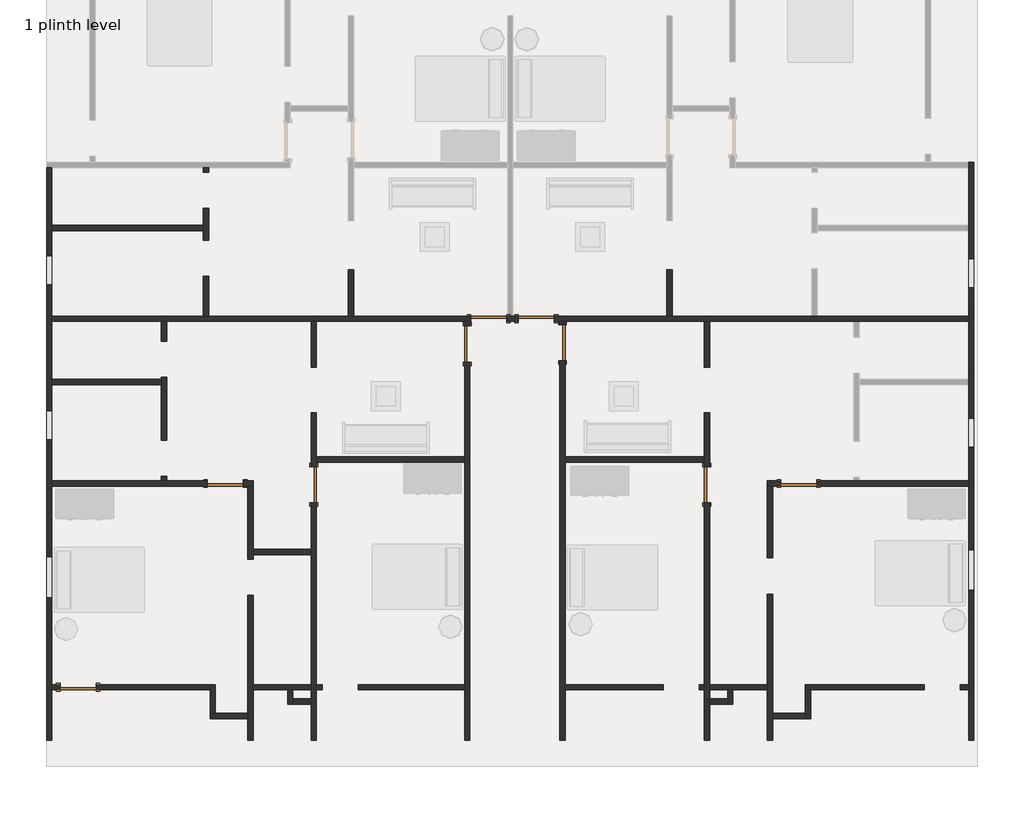
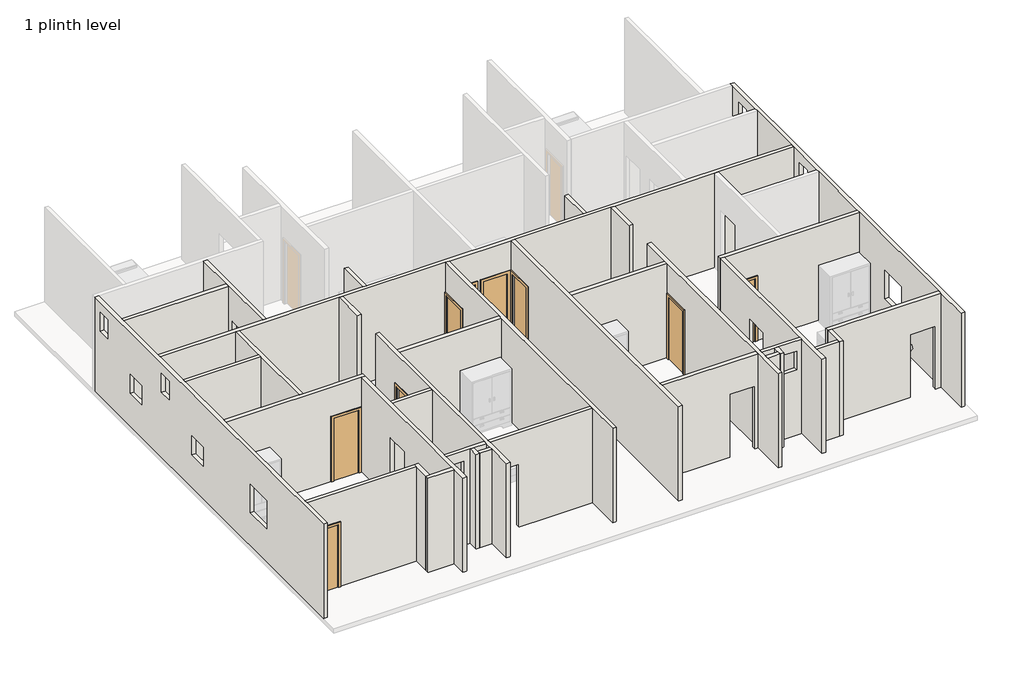
# One storey, part 1 of 2: 36 walls, 9 doors.
"""IFC4 building model written with IfcOpenShell, lengths in millimetres."""

from ifc_helpers import new_model, si_unit, frame, origin, place, context, project, spatial, polyline, outline, extrude, faceted_brep, transform, mapped, element, save
from components import door_f2b275c1, door_d8f5dbb5

model = new_model("IFC4")

# Units and contexts
model_context = context("Model", 3, world=origin())
ifc_project = project(units=[si_unit("LENGTHUNIT", "METRE", prefix="MILLI")], contexts=[model_context])

# Site, building, storey
site = spatial("IfcSite", under=ifc_project)
building = spatial("IfcBuilding", under=site)
storey = spatial("IfcBuildingStorey", under=building, Name="1 plinth level", Elevation=457.2)

# Doors
placement = place(None, origin())
door_shape = door_f2b275c1(model_context)
element("IfcDoor", 1, ObjectType="Single-Flush : 30\" x 80\"", at=placement, inside=storey, context=model_context, shape_type="MappedRepresentation", body=[
    mapped(door_shape, transform((-4502.7689207, -2247.7064399, 457.2), x_axis=(-1.0, 0.0, 0.0), y_axis=(0.0, -1.0, 0.0), z_axis=(0.0, 0.0, 1.0))),
])
element("IfcDoor", 2, ObjectType="Single-Flush : 30\" x 80\"", at=placement, inside=storey, context=model_context, shape_type="MappedRepresentation", body=[
    mapped(door_shape, transform((-3950.4035225, -2755.7064399, 457.2), x_axis=(0.0, 1.0, 0.0), y_axis=(-1.0, 0.0, 0.0), z_axis=(0.0, 0.0, 1.0))),
])
element("IfcDoor", 3, ObjectType="Single-Flush : 30\" x 80\"", at=placement, inside=storey, context=model_context, shape_type="MappedRepresentation", body=[
    mapped(door_shape, transform((-11074.9343188, -5727.5064399, 457.2), x_axis=(1.0, 0.0, 0.0), y_axis=(0.0, 1.0, 0.0), z_axis=(0.0, 0.0, 1.0))),
])
element("IfcDoor", 4, ObjectType="Single-Flush : 30\" x 80\"", at=placement, inside=storey, context=model_context, shape_type="MappedRepresentation", body=[
    mapped(door_shape, transform((-9208.0343188, -5752.9064399, 457.2), x_axis=(0.0, 1.0, 0.0), y_axis=(-1.0, 0.0, 0.0), z_axis=(0.0, 0.0, 1.0))),
])
door_2_shape = door_d8f5dbb5(model_context)
element("IfcDoor", 5, ObjectType="Single-Flush : 30\" x 80\"", at=placement, inside=storey, context=model_context, shape_type="MappedRepresentation", body=[
    mapped(door_2_shape, transform((-5509.7738197, -2247.7064399, 457.2), x_axis=(1.0, 0.0, 0.0), y_axis=(0.0, 1.0, 0.0), z_axis=(0.0, 0.0, 1.0))),
])
element("IfcDoor", 6, ObjectType="Single-Flush : 30\" x 80\"", at=placement, inside=storey, context=model_context, shape_type="MappedRepresentation", body=[
    mapped(door_2_shape, transform((-5964.4133206, -2781.1064399, 457.2), x_axis=(0.0, 1.0, 0.0), y_axis=(-1.0, 0.0, 0.0), z_axis=(0.0, 0.0, 1.0))),
])
element("IfcDoor", 7, ObjectType="Single-Flush : 30\" x 80\"", at=placement, inside=storey, context=model_context, shape_type="MappedRepresentation", body=[
    mapped(door_2_shape, transform((1040.8656812, -5727.5064399, 457.2), x_axis=(-1.0, 0.0, 0.0), y_axis=(0.0, -1.0, 0.0), z_axis=(0.0, 0.0, 1.0))),
])
element("IfcDoor", 8, ObjectType="Single-Flush : 30\" x 80\"", at=placement, inside=storey, context=model_context, shape_type="MappedRepresentation", body=[
    mapped(door_2_shape, transform((-902.2343188, -5755.6106007, 457.2), x_axis=(0.0, 1.0, 0.0), y_axis=(-1.0, 0.0, 0.0), z_axis=(0.0, 0.0, 1.0))),
])
element("IfcDoor", 9, ObjectType="Single-Flush : 30\" x 80\"", at=placement, inside=storey, context=model_context, shape_type="MappedRepresentation", body=[
    mapped(door_2_shape, transform((-14186.4343188, -10032.8064399, 457.2), x_axis=(-1.0, 0.0, 0.0), y_axis=(0.0, -1.0, 0.0), z_axis=(0.0, 0.0, 1.0))),
])

# Walls
element("IfcWall", 10, ObjectType="wall-4.5\"", at=placement, inside=storey, context=model_context, shape_type="Brep", body=[
    faceted_brep([(4628.6156812, 1060.6435601, 457.2), (4628.6156812, 946.3435601, 457.2), (4628.6156812, -272.8564399, 457.2), (4628.6156812, -387.1564399, 457.2), (4628.6156812, -2190.5564399, 457.2), (4628.6156812, -2304.8564399, 457.2), (4628.6156812, -3524.0564399, 457.2), (4628.6156812, -3638.3564399, 457.2), (4628.6156812, -5670.3564399, 457.2), (4628.6156812, -5784.6564399, 457.2), (4628.6156812, -9975.6564399, 457.2), (4628.6156812, -10089.9564399, 457.2), (4628.6156812, -11156.7564399, 457.2), (4628.6156812, -11156.7564399, 3505.2), (4628.6156812, -10089.9564399, 3505.2), (4628.6156812, -9975.6564399, 3505.2), (4628.6156812, -5784.6564399, 3505.2), (4628.6156812, -5670.3564399, 3505.2), (4628.6156812, -3638.3564399, 3505.2), (4628.6156812, -3524.0564399, 3505.2), (4628.6156812, -2304.8564399, 3505.2), (4628.6156812, -2190.5564399, 3505.2), (4628.6156812, -387.1564399, 3505.2), (4628.6156812, -272.8564399, 3505.2), (4628.6156812, 946.3435601, 3505.2), (4628.6156812, 1060.6435601, 3505.2), (4628.6156812, -7988.1064399, 2438.4), (4628.6156812, -7988.1064399, 1524.0), (4628.6156812, -7124.5064399, 1524.0), (4628.6156812, -7124.5064399, 2438.4), (4628.6156812, -2603.3064399, 3175.0), (4628.6156812, -3009.7064399, 3175.0), (4628.6156812, -3009.7064399, 2565.4), (4628.6156812, -2603.3064399, 2565.4), (4628.6156812, 622.4935601, 3175.0), (4628.6156812, 216.0935601, 3175.0), (4628.6156812, 216.0935601, 2565.4), (4628.6156812, 622.4935601, 2565.4), (4628.6156812, -984.0564399, 2133.6), (4628.6156812, -1593.6564399, 2133.6), (4628.6156812, -1593.6564399, 1524.0), (4628.6156812, -984.0564399, 1524.0), (4628.6156812, -4959.1564399, 2133.6), (4628.6156812, -4959.1564399, 1524.0), (4628.6156812, -4349.5564399, 1524.0), (4628.6156812, -4349.5564399, 2133.6), (4742.9156812, 1060.6435601, 457.2), (4742.9156812, 1060.6435601, 3505.2), (4742.9156812, -11156.7564399, 3505.2), (4742.9156812, -11156.7564399, 457.2), (4742.9156812, -7988.1064399, 2438.4), (4742.9156812, -7124.5064399, 2438.4), (4742.9156812, -7124.5064399, 1524.0), (4742.9156812, -7988.1064399, 1524.0), (4742.9156812, -2603.3064399, 3175.0), (4742.9156812, -2603.3064399, 2565.4), (4742.9156812, -3009.7064399, 2565.4), (4742.9156812, -3009.7064399, 3175.0), (4742.9156812, 622.4935601, 3175.0), (4742.9156812, 622.4935601, 2565.4), (4742.9156812, 216.0935601, 2565.4), (4742.9156812, 216.0935601, 3175.0), (4742.9156812, -984.0564399, 2133.6), (4742.9156812, -984.0564399, 1524.0), (4742.9156812, -1593.6564399, 1524.0), (4742.9156812, -1593.6564399, 2133.6), (4742.9156812, -4959.1564399, 2133.6), (4742.9156812, -4349.5564399, 2133.6), (4742.9156812, -4349.5564399, 1524.0), (4742.9156812, -4959.1564399, 1524.0)], [[[0, 1, 2, 3, 4, 5, 6, 7, 8, 9, 10, 11, 12, 13, 14, 15, 16, 17, 18, 19, 20, 21, 22, 23, 24, 25], [26, 27, 28, 29], [30, 31, 32, 33], [34, 35, 36, 37], [38, 39, 40, 41], [42, 43, 44, 45]], [[46, 47, 48, 49], [50, 51, 52, 53], [54, 55, 56, 57], [58, 59, 60, 61], [62, 63, 64, 65], [66, 67, 68, 69]], [[12, 11, 10, 9, 8, 7, 6, 5, 4, 3, 2, 1, 0, 46, 49]], [[13, 12, 49, 48]], [[25, 24, 23, 22, 21, 20, 19, 18, 17, 16, 15, 14, 13, 48, 47]], [[0, 25, 47, 46]], [[27, 26, 50, 53]], [[28, 27, 53, 52]], [[29, 28, 52, 51]], [[26, 29, 51, 50]], [[55, 54, 30, 33]], [[56, 55, 33, 32]], [[57, 56, 32, 31]], [[54, 57, 31, 30]], [[59, 58, 34, 37]], [[60, 59, 37, 36]], [[61, 60, 36, 35]], [[58, 61, 35, 34]], [[63, 62, 38, 41]], [[64, 63, 41, 40]], [[65, 64, 40, 39]], [[62, 65, 39, 38]], [[43, 42, 66, 69]], [[44, 43, 69, 68]], [[45, 44, 68, 67]], [[42, 45, 67, 66]]]),
])
element("IfcWall", 11, ObjectType="wall-4.5\"", at=placement, inside=storey, context=model_context, shape_type="Brep", body=[
    faceted_brep([(-14853.1843188, 946.3435601, 457.2), (-14853.1843188, -11156.7564399, 457.2), (-14853.1843188, -11156.7564399, 3505.2), (-14853.1843188, 946.3435601, 3505.2), (-14853.1843188, -7276.9064399, 2438.4), (-14853.1843188, -8140.5064399, 2438.4), (-14853.1843188, -8140.5064399, 1524.0), (-14853.1843188, -7276.9064399, 1524.0), (-14853.1843188, 266.8935601, 3175.0), (-14853.1843188, 266.8935601, 2565.4), (-14853.1843188, 673.2935601, 2565.4), (-14853.1843188, 673.2935601, 3175.0), (-14853.1843188, -2577.9064399, 3175.0), (-14853.1843188, -2984.3064399, 3175.0), (-14853.1843188, -2984.3064399, 2565.4), (-14853.1843188, -2577.9064399, 2565.4), (-14853.1843188, -1523.8064399, 2133.6), (-14853.1843188, -1523.8064399, 1524.0), (-14853.1843188, -914.2064399, 1524.0), (-14853.1843188, -914.2064399, 2133.6), (-14853.1843188, -4190.8064399, 2133.6), (-14853.1843188, -4800.4064399, 2133.6), (-14853.1843188, -4800.4064399, 1524.0), (-14853.1843188, -4190.8064399, 1524.0), (-14738.8843188, 946.3435601, 457.2), (-14738.8843188, 946.3435601, 3505.2), (-14738.8843188, -272.8564399, 3505.2), (-14738.8843188, -387.1564399, 3505.2), (-14738.8843188, -2190.5564399, 3505.2), (-14738.8843188, -2304.8564399, 3505.2), (-14738.8843188, -3524.0564399, 3505.2), (-14738.8843188, -3638.3564399, 3505.2), (-14738.8843188, -5670.3564399, 3505.2), (-14738.8843188, -5784.6564399, 3505.2), (-14738.8843188, -9975.6564399, 3505.2), (-14738.8843188, -10089.9564399, 3505.2), (-14738.8843188, -11156.7564399, 3505.2), (-14738.8843188, -11156.7564399, 457.2), (-14738.8843188, -10089.9564399, 457.2), (-14738.8843188, -9975.6564399, 457.2), (-14738.8843188, -5784.6564399, 457.2), (-14738.8843188, -5670.3564399, 457.2), (-14738.8843188, -3638.3564399, 457.2), (-14738.8843188, -3524.0564399, 457.2), (-14738.8843188, -2304.8564399, 457.2), (-14738.8843188, -2190.5564399, 457.2), (-14738.8843188, -387.1564399, 457.2), (-14738.8843188, -272.8564399, 457.2), (-14738.8843188, -7276.9064399, 2438.4), (-14738.8843188, -7276.9064399, 1524.0), (-14738.8843188, -8140.5064399, 1524.0), (-14738.8843188, -8140.5064399, 2438.4), (-14738.8843188, 266.8935601, 3175.0), (-14738.8843188, 673.2935601, 3175.0), (-14738.8843188, 673.2935601, 2565.4), (-14738.8843188, 266.8935601, 2565.4), (-14738.8843188, -2577.9064399, 3175.0), (-14738.8843188, -2577.9064399, 2565.4), (-14738.8843188, -2984.3064399, 2565.4), (-14738.8843188, -2984.3064399, 3175.0), (-14738.8843188, -1523.8064399, 2133.6), (-14738.8843188, -914.2064399, 2133.6), (-14738.8843188, -914.2064399, 1524.0), (-14738.8843188, -1523.8064399, 1524.0), (-14738.8843188, -4190.8064399, 2133.6), (-14738.8843188, -4190.8064399, 1524.0), (-14738.8843188, -4800.4064399, 1524.0), (-14738.8843188, -4800.4064399, 2133.6)], [[[0, 1, 2, 3], [4, 5, 6, 7], [8, 9, 10, 11], [12, 13, 14, 15], [16, 17, 18, 19], [20, 21, 22, 23]], [[24, 25, 26, 27, 28, 29, 30, 31, 32, 33, 34, 35, 36, 37, 38, 39, 40, 41, 42, 43, 44, 45, 46, 47], [48, 49, 50, 51], [52, 53, 54, 55], [56, 57, 58, 59], [60, 61, 62, 63], [64, 65, 66, 67]], [[1, 0, 24, 47, 46, 45, 44, 43, 42, 41, 40, 39, 38, 37]], [[2, 1, 37, 36]], [[3, 2, 36, 35, 34, 33, 32, 31, 30, 29, 28, 27, 26, 25]], [[0, 3, 25, 24]], [[49, 48, 4, 7]], [[50, 49, 7, 6]], [[51, 50, 6, 5]], [[48, 51, 5, 4]], [[9, 8, 52, 55]], [[10, 9, 55, 54]], [[11, 10, 54, 53]], [[8, 11, 53, 52]], [[57, 56, 12, 15]], [[58, 57, 15, 14]], [[59, 58, 14, 13]], [[56, 59, 13, 12]], [[17, 16, 60, 63]], [[18, 17, 63, 62]], [[19, 18, 62, 61]], [[16, 19, 61, 60]], [[65, 64, 20, 23]], [[66, 65, 23, 22]], [[67, 66, 22, 21]], [[64, 67, 21, 20]]]),
])
element("IfcWall", 12, ObjectType="wall-4.5\"", at=placement, inside=storey, context=model_context, shape_type="Brep", body=[
    faceted_brep([(-11538.4843188, 946.3435601, 457.2), (-11538.4843188, 851.0935601, 457.2), (-11538.4843188, 851.0935601, 2489.2), (-11538.4843188, 89.0935601, 2489.2), (-11538.4843188, 89.0935601, 457.2), (-11538.4843188, -272.8564399, 457.2), (-11538.4843188, -387.1564399, 457.2), (-11538.4843188, -584.0064399, 457.2), (-11538.4843188, -584.0064399, 2489.2), (-11538.4843188, -1346.0064399, 2489.2), (-11538.4843188, -1346.0064399, 457.2), (-11538.4843188, -2190.5564399, 457.2), (-11538.4843188, -2190.5564399, 3505.2), (-11538.4843188, -387.1564399, 3505.2), (-11538.4843188, -272.8564399, 3505.2), (-11538.4843188, 946.3435601, 3505.2), (-11424.1843188, 851.0935601, 2489.2), (-11424.1843188, 851.0935601, 457.2), (-11424.1843188, 946.3435601, 457.2), (-11424.1843188, 946.3435601, 3505.2), (-11424.1843188, -2190.5564399, 3505.2), (-11424.1843188, -2190.5564399, 457.2), (-11424.1843188, -1346.0064399, 457.2), (-11424.1843188, -1346.0064399, 2489.2), (-11424.1843188, -584.0064399, 2489.2), (-11424.1843188, -584.0064399, 457.2), (-11424.1843188, 89.0935601, 457.2), (-11424.1843188, 89.0935601, 2489.2)], [[[0, 1, 2, 3, 4, 5, 6, 7, 8, 9, 10, 11, 12, 13, 14, 15]], [[16, 17, 18, 19, 20, 21, 22, 23, 24, 25, 26, 27]], [[22, 21, 11, 10]], [[26, 25, 7, 6, 5, 4]], [[18, 17, 1, 0]], [[15, 14, 13, 12, 20, 19]], [[0, 15, 19, 18]], [[12, 11, 21, 20]], [[8, 7, 25, 24]], [[9, 8, 24, 23]], [[10, 9, 23, 22]], [[2, 1, 17, 16]], [[3, 2, 16, 27]], [[4, 3, 27, 26]]]),
])
element("IfcWall", 13, ObjectType="wall-4.5\"", at=placement, inside=storey, context=model_context, shape_type="SweptSolid", body=[
    extrude(outline(polyline([(-11538.4843188, -387.1564399), (-14738.8843188, -387.1564399), (-14738.8843188, -272.8564399), (-11538.4843188, -272.8564399), (-11538.4843188, -387.1564399)])), frame((0.0, 0.0, 457.2), z_axis=(0.0, 0.0, 1.0), x_axis=(1.0, 0.0, 0.0)), (0.0, 0.0, 1.0), 3048.0),
])
element("IfcWall", 14, ObjectType="wall-4.5\"", at=placement, inside=storey, context=model_context, shape_type="Brep", body=[
    faceted_brep([(-12427.4843188, -3479.6064399, 2489.2), (-12427.4843188, -3479.6064399, 457.2), (-12427.4843188, -3524.0564399, 457.2), (-12427.4843188, -3638.3564399, 457.2), (-12427.4843188, -4813.1064399, 457.2), (-12427.4843188, -4813.1064399, 2489.2), (-12427.4843188, -5575.1064399, 2489.2), (-12427.4843188, -5575.1064399, 457.2), (-12427.4843188, -5670.3564399, 457.2), (-12427.4843188, -5670.3564399, 3505.2), (-12427.4843188, -3638.3564399, 3505.2), (-12427.4843188, -3524.0564399, 3505.2), (-12427.4843188, -2304.8564399, 3505.2), (-12427.4843188, -2304.8564399, 457.2), (-12427.4843188, -2717.6064399, 457.2), (-12427.4843188, -2717.6064399, 2489.2), (-12313.1843188, -4813.1064399, 457.2), (-12313.1843188, -3479.6064399, 457.2), (-12313.1843188, -3479.6064399, 2489.2), (-12313.1843188, -2717.6064399, 2489.2), (-12313.1843188, -2717.6064399, 457.2), (-12313.1843188, -2304.8564399, 457.2), (-12313.1843188, -2304.8564399, 3505.2), (-12313.1843188, -5670.3564399, 3505.2), (-12313.1843188, -5670.3564399, 457.2), (-12313.1843188, -5575.1064399, 457.2), (-12313.1843188, -5575.1064399, 2489.2), (-12313.1843188, -4813.1064399, 2489.2)], [[[0, 1, 2, 3, 4, 5, 6, 7, 8, 9, 10, 11, 12, 13, 14, 15]], [[16, 17, 18, 19, 20, 21, 22, 23, 24, 25, 26, 27]], [[8, 7, 25, 24]], [[14, 13, 21, 20]], [[4, 3, 2, 1, 17, 16]], [[12, 11, 10, 9, 23, 22]], [[13, 12, 22, 21]], [[9, 8, 24, 23]], [[26, 25, 7, 6]], [[27, 26, 6, 5]], [[16, 27, 5, 4]], [[18, 17, 1, 0]], [[19, 18, 0, 15]], [[20, 19, 15, 14]]]),
])
element("IfcWall", 15, ObjectType="wall-4.5\"", at=placement, inside=storey, context=model_context, shape_type="Brep", body=[
    faceted_brep([(-10484.3843188, -5784.6564399, 3505.2), (-10598.6843188, -5784.6564399, 3505.2), (-14738.8843188, -5784.6564399, 3505.2), (-14738.8843188, -5784.6564399, 457.2), (-11455.9343188, -5784.6564399, 457.2), (-11455.9343188, -5784.6564399, 2489.2), (-10693.9343188, -5784.6564399, 2489.2), (-10693.9343188, -5784.6564399, 457.2), (-10598.6843188, -5784.6564399, 457.2), (-10484.3843188, -5784.6564399, 457.2), (-14738.8843188, -5670.3564399, 3505.2), (-12427.4843188, -5670.3564399, 3505.2), (-12313.1843188, -5670.3564399, 3505.2), (-10484.3843188, -5670.3564399, 3505.2), (-10484.3843188, -5670.3564399, 457.2), (-10693.9343188, -5670.3564399, 457.2), (-10693.9343188, -5670.3564399, 2489.2), (-11455.9343188, -5670.3564399, 2489.2), (-11455.9343188, -5670.3564399, 457.2), (-12313.1843188, -5670.3564399, 457.2), (-12427.4843188, -5670.3564399, 457.2), (-14738.8843188, -5670.3564399, 457.2)], [[[0, 1, 2, 3, 4, 5, 6, 7, 8, 9]], [[10, 11, 12, 13, 14, 15, 16, 17, 18, 19, 20, 21]], [[3, 21, 20, 19, 18, 4]], [[14, 9, 8, 7, 15]], [[2, 1, 0, 13, 12, 11, 10]], [[3, 2, 10, 21]], [[0, 9, 14, 13]], [[6, 16, 15, 7]], [[16, 6, 5, 17]], [[17, 5, 4, 18]]]),
])
element("IfcWall", 16, ObjectType="wall-4.5\"", at=placement, inside=storey, context=model_context, shape_type="SweptSolid", body=[
    extrude(outline(polyline([(3505.2, -11398.7843188), (3505.2, -14738.8843188), (457.2, -14738.8843188), (457.2, -14567.4343188), (2489.2, -14567.4343188), (2489.2, -13805.4343188), (457.2, -13805.4343188), (457.2, -11398.7843188), (3505.2, -11398.7843188)])), frame((0.0, -10089.9564399, 0.0), z_axis=(0.0, 1.0, 0.0), x_axis=(0.0, 0.0, 1.0)), (0.0, 0.0, 1.0), 114.3),
])
element("IfcWall", 17, ObjectType="wall-4.5\"", at=placement, inside=storey, context=model_context, shape_type="Brep", body=[
    faceted_brep([(-11398.7843188, -9975.6564399, 457.2), (-11398.7843188, -10089.9564399, 457.2), (-11398.7843188, -10585.2564399, 457.2), (-11398.7843188, -10585.2564399, 3505.2), (-11398.7843188, -10089.9564399, 3505.2), (-11398.7843188, -9975.6564399, 3505.2), (-11284.4843188, -9975.6564399, 457.2), (-11284.4843188, -9975.6564399, 3505.2), (-11284.4843188, -10585.2564399, 3505.2), (-11284.4843188, -10585.2564399, 457.2)], [[[0, 1, 2, 3, 4, 5]], [[6, 7, 8, 9]], [[2, 1, 0, 6, 9]], [[5, 4, 3, 8, 7]], [[3, 2, 9, 8]], [[0, 5, 7, 6]]]),
])
element("IfcWall", 18, ObjectType="wall-4.5\"", at=placement, inside=storey, context=model_context, shape_type="Brep", body=[
    faceted_brep([(-10598.6843188, -10585.2564399, 457.2), (-11284.4843188, -10585.2564399, 457.2), (-11398.7843188, -10585.2564399, 457.2), (-11398.7843188, -10585.2564399, 3505.2), (-11284.4843188, -10585.2564399, 3505.2), (-10598.6843188, -10585.2564399, 3505.2), (-10598.6843188, -10699.5564399, 457.2), (-10598.6843188, -10699.5564399, 3505.2), (-11398.7843188, -10699.5564399, 3505.2), (-11398.7843188, -10699.5564399, 457.2)], [[[0, 1, 2, 3, 4, 5]], [[6, 7, 8, 9]], [[2, 1, 0, 6, 9]], [[5, 4, 3, 8, 7]], [[0, 5, 7, 6]], [[3, 2, 9, 8]]]),
])
element("IfcWall", 19, ObjectType="wall-4.5\"", at=placement, inside=storey, context=model_context, shape_type="Brep", body=[
    faceted_brep([(-10484.3843188, -7327.7064399, 2489.2), (-10484.3843188, -7327.7064399, 457.2), (-10484.3843188, -7232.4564399, 457.2), (-10484.3843188, -7118.1564399, 457.2), (-10484.3843188, -5784.6564399, 457.2), (-10484.3843188, -5784.6564399, 3505.2), (-10484.3843188, -7118.1564399, 3505.2), (-10484.3843188, -7232.4564399, 3505.2), (-10484.3843188, -9975.6564399, 3505.2), (-10484.3843188, -10089.9564399, 3505.2), (-10484.3843188, -11156.7564399, 3505.2), (-10484.3843188, -11156.7564399, 457.2), (-10484.3843188, -10089.9564399, 457.2), (-10484.3843188, -9975.6564399, 457.2), (-10484.3843188, -8089.7064399, 457.2), (-10484.3843188, -8089.7064399, 2489.2), (-10598.6843188, -5784.6564399, 457.2), (-10598.6843188, -7327.7064399, 457.2), (-10598.6843188, -7327.7064399, 2489.2), (-10598.6843188, -8089.7064399, 2489.2), (-10598.6843188, -8089.7064399, 457.2), (-10598.6843188, -10585.2564399, 457.2), (-10598.6843188, -10699.5564399, 457.2), (-10598.6843188, -11156.7564399, 457.2), (-10598.6843188, -11156.7564399, 3505.2), (-10598.6843188, -10699.5564399, 3505.2), (-10598.6843188, -10585.2564399, 3505.2), (-10598.6843188, -5784.6564399, 3505.2)], [[[0, 1, 2, 3, 4, 5, 6, 7, 8, 9, 10, 11, 12, 13, 14, 15]], [[16, 17, 18, 19, 20, 21, 22, 23, 24, 25, 26, 27]], [[14, 13, 12, 11, 23, 22, 21, 20]], [[4, 3, 2, 1, 17, 16]], [[10, 9, 8, 7, 6, 5, 27, 26, 25, 24]], [[11, 10, 24, 23]], [[5, 4, 16, 27]], [[18, 17, 1, 0]], [[19, 18, 0, 15]], [[20, 19, 15, 14]]]),
])
element("IfcWall", 20, ObjectType="wall-4.5\"", at=placement, inside=storey, context=model_context, shape_type="Brep", body=[
    faceted_brep([(4628.6156812, -2304.8564399, 3505.2), (2317.2156812, -2304.8564399, 3505.2), (2202.9156812, -2304.8564399, 3505.2), (-845.0843188, -2304.8564399, 3505.2), (-959.3843188, -2304.8564399, 3505.2), (-3893.2535225, -2304.8564399, 3505.2), (-4007.5535225, -2304.8564399, 3505.2), (-5907.2633206, -2304.8564399, 3505.2), (-6021.5633206, -2304.8564399, 3505.2), (-9150.8843188, -2304.8564399, 3505.2), (-9265.1843188, -2304.8564399, 3505.2), (-12313.1843188, -2304.8564399, 3505.2), (-12427.4843188, -2304.8564399, 3505.2), (-14738.8843188, -2304.8564399, 3505.2), (-14738.8843188, -2304.8564399, 457.2), (-12427.4843188, -2304.8564399, 457.2), (-12313.1843188, -2304.8564399, 457.2), (-9265.1843188, -2304.8564399, 457.2), (-9150.8843188, -2304.8564399, 457.2), (-6021.5633206, -2304.8564399, 457.2), (-5907.2633206, -2304.8564399, 457.2), (-5890.7738197, -2304.8564399, 457.2), (-5890.7738197, -2304.8564399, 2489.2), (-5128.7738197, -2304.8564399, 2489.2), (-5128.7738197, -2304.8564399, 457.2), (-4883.7689207, -2304.8564399, 457.2), (-4883.7689207, -2304.8564399, 2489.2), (-4121.7689207, -2304.8564399, 2489.2), (-4121.7689207, -2304.8564399, 457.2), (-4007.5535225, -2304.8564399, 457.2), (-3893.2535225, -2304.8564399, 457.2), (-959.3843188, -2304.8564399, 457.2), (-845.0843188, -2304.8564399, 457.2), (2202.9156812, -2304.8564399, 457.2), (2317.2156812, -2304.8564399, 457.2), (4628.6156812, -2304.8564399, 457.2), (-14738.8843188, -2190.5564399, 3505.2), (-11538.4843188, -2190.5564399, 3505.2), (-11424.1843188, -2190.5564399, 3505.2), (-8477.7843188, -2190.5564399, 3505.2), (-8363.4843188, -2190.5564399, 3505.2), (-5112.2843188, -2190.5564399, 3505.2), (-4997.9843188, -2190.5564399, 3505.2), (-1746.7843188, -2190.5564399, 3505.2), (-1632.4843188, -2190.5564399, 3505.2), (1313.9156812, -2190.5564399, 3505.2), (1428.2156812, -2190.5564399, 3505.2), (4628.6156812, -2190.5564399, 3505.2), (4628.6156812, -2190.5564399, 457.2), (1428.2156812, -2190.5564399, 457.2), (1313.9156812, -2190.5564399, 457.2), (-1632.4843188, -2190.5564399, 457.2), (-1746.7843188, -2190.5564399, 457.2), (-4121.7689207, -2190.5564399, 457.2), (-4121.7689207, -2190.5564399, 2489.2), (-4883.7689207, -2190.5564399, 2489.2), (-4883.7689207, -2190.5564399, 457.2), (-4997.9843188, -2190.5564399, 457.2), (-5112.2843188, -2190.5564399, 457.2), (-5128.7738197, -2190.5564399, 457.2), (-5128.7738197, -2190.5564399, 2489.2), (-5890.7738197, -2190.5564399, 2489.2), (-5890.7738197, -2190.5564399, 457.2), (-8363.4843188, -2190.5564399, 457.2), (-8477.7843188, -2190.5564399, 457.2), (-11424.1843188, -2190.5564399, 457.2), (-11538.4843188, -2190.5564399, 457.2), (-14738.8843188, -2190.5564399, 457.2)], [[[0, 1, 2, 3, 4, 5, 6, 7, 8, 9, 10, 11, 12, 13, 14, 15, 16, 17, 18, 19, 20, 21, 22, 23, 24, 25, 26, 27, 28, 29, 30, 31, 32, 33, 34, 35]], [[36, 37, 38, 39, 40, 41, 42, 43, 44, 45, 46, 47, 48, 49, 50, 51, 52, 53, 54, 55, 56, 57, 58, 59, 60, 61, 62, 63, 64, 65, 66, 67]], [[14, 67, 66, 65, 64, 63, 62, 21, 20, 19, 18, 17, 16, 15]], [[48, 35, 34, 33, 32, 31, 30, 29, 28, 53, 52, 51, 50, 49]], [[56, 25, 24, 59, 58, 57]], [[13, 12, 11, 10, 9, 8, 7, 6, 5, 4, 3, 2, 1, 0, 47, 46, 45, 44, 43, 42, 41, 40, 39, 38, 37, 36]], [[0, 35, 48, 47]], [[14, 13, 36, 67]], [[55, 26, 25, 56]], [[26, 55, 54, 27]], [[27, 54, 53, 28]], [[23, 60, 59, 24]], [[60, 23, 22, 61]], [[61, 22, 21, 62]]]),
])
element("IfcWall", 21, ObjectType="wall-4.5\"", at=placement, inside=storey, context=model_context, shape_type="SweptSolid", body=[
    extrude(outline(polyline([(-8363.4843188, -1214.893875), (-8363.4843188, -2190.5564399), (-8477.7843188, -2190.5564399), (-8477.7843188, -1214.893875), (-8363.4843188, -1214.893875)])), frame((0.0, 0.0, 457.2), z_axis=(0.0, 0.0, 1.0), x_axis=(1.0, 0.0, 0.0)), (0.0, 0.0, 1.0), 3048.0),
])
element("IfcWall", 22, ObjectType="wall-4.5\"", at=placement, inside=storey, context=model_context, shape_type="SweptSolid", body=[
    extrude(outline(polyline([(-9265.1843188, -3270.1509299), (-9265.1843188, -2304.8564399), (-9150.8843188, -2304.8564399), (-9150.8843188, -3270.1509299), (-9265.1843188, -3270.1509299)])), frame((0.0, 0.0, 457.2), z_axis=(0.0, 0.0, 1.0), x_axis=(1.0, 0.0, 0.0)), (0.0, 0.0, 1.0), 3048.0),
])
element("IfcWall", 23, ObjectType="wall-4.5\"", at=placement, inside=storey, context=model_context, shape_type="SweptSolid", body=[
    extrude(outline(polyline([(-1632.4843188, -1214.893875), (-1632.4843188, -2190.5564399), (-1746.7843188, -2190.5564399), (-1746.7843188, -1214.893875), (-1632.4843188, -1214.893875)])), frame((0.0, 0.0, 457.2), z_axis=(0.0, 0.0, 1.0), x_axis=(1.0, 0.0, 0.0)), (0.0, 0.0, 1.0), 3048.0),
])
element("IfcWall", 24, ObjectType="wall-4.5\"", at=placement, inside=storey, context=model_context, shape_type="SweptSolid", body=[
    extrude(outline(polyline([(-959.3843188, -3270.1509299), (-959.3843188, -2304.8564399), (-845.0843188, -2304.8564399), (-845.0843188, -3270.1509299), (-959.3843188, -3270.1509299)])), frame((0.0, 0.0, 457.2), z_axis=(0.0, 0.0, 1.0), x_axis=(1.0, 0.0, 0.0)), (0.0, 0.0, 1.0), 3048.0),
])
element("IfcWall", 25, ObjectType="wall-4.5\"", at=placement, inside=storey, context=model_context, shape_type="Brep", body=[
    faceted_brep([(-6021.5633206, -11156.7564399, 457.2), (-6021.5633206, -11156.7564399, 3505.2), (-6021.5633206, -10089.9564399, 3505.2), (-6021.5633206, -9975.6564399, 3505.2), (-6021.5633206, -5276.6564399, 3505.2), (-6021.5633206, -5162.3564399, 3505.2), (-6021.5633206, -2304.8564399, 3505.2), (-6021.5633206, -2304.8564399, 457.2), (-6021.5633206, -2400.1064399, 457.2), (-6021.5633206, -2400.1064399, 2489.2), (-6021.5633206, -3162.1064399, 2489.2), (-6021.5633206, -3162.1064399, 457.2), (-6021.5633206, -5162.3564399, 457.2), (-6021.5633206, -5276.6564399, 457.2), (-6021.5633206, -9975.6564399, 457.2), (-6021.5633206, -10089.9564399, 457.2), (-5907.2633206, -11156.7564399, 3505.2), (-5907.2633206, -11156.7564399, 457.2), (-5907.2633206, -3162.1064399, 457.2), (-5907.2633206, -3162.1064399, 2489.2), (-5907.2633206, -2400.1064399, 2489.2), (-5907.2633206, -2400.1064399, 457.2), (-5907.2633206, -2304.8564399, 457.2), (-5907.2633206, -2304.8564399, 3505.2)], [[[0, 1, 2, 3, 4, 5, 6, 7, 8, 9, 10, 11, 12, 13, 14, 15]], [[16, 17, 18, 19, 20, 21, 22, 23]], [[17, 0, 15, 14, 13, 12, 11, 18]], [[7, 22, 21, 8]], [[1, 0, 17, 16]], [[6, 5, 4, 3, 2, 1, 16, 23]], [[7, 6, 23, 22]], [[20, 9, 8, 21]], [[9, 20, 19, 10]], [[10, 19, 18, 11]]]),
])
element("IfcWall", 26, ObjectType="wall-4.5\"", at=placement, inside=storey, context=model_context, shape_type="Brep", body=[
    faceted_brep([(-3893.2535225, -2304.8564399, 3505.2), (-3893.2535225, -5162.3564399, 3505.2), (-3893.2535225, -5276.6564399, 3505.2), (-3893.2535225, -9975.6564399, 3505.2), (-3893.2535225, -10089.9564399, 3505.2), (-3893.2535225, -11156.7564399, 3505.2), (-3893.2535225, -11156.7564399, 457.2), (-3893.2535225, -10089.9564399, 457.2), (-3893.2535225, -9975.6564399, 457.2), (-3893.2535225, -5276.6564399, 457.2), (-3893.2535225, -5162.3564399, 457.2), (-3893.2535225, -3136.7064399, 457.2), (-3893.2535225, -3136.7064399, 2489.2), (-3893.2535225, -2374.7064399, 2489.2), (-3893.2535225, -2374.7064399, 457.2), (-3893.2535225, -2304.8564399, 457.2), (-4007.5535225, -11156.7564399, 3505.2), (-4007.5535225, -2304.8564399, 3505.2), (-4007.5535225, -2304.8564399, 457.2), (-4007.5535225, -2374.7064399, 457.2), (-4007.5535225, -2374.7064399, 2489.2), (-4007.5535225, -3136.7064399, 2489.2), (-4007.5535225, -3136.7064399, 457.2), (-4007.5535225, -11156.7564399, 457.2)], [[[0, 1, 2, 3, 4, 5, 6, 7, 8, 9, 10, 11, 12, 13, 14, 15]], [[16, 17, 18, 19, 20, 21, 22, 23]], [[6, 23, 22, 11, 10, 9, 8, 7]], [[18, 15, 14, 19]], [[5, 4, 3, 2, 1, 0, 17, 16]], [[6, 5, 16, 23]], [[0, 15, 18, 17]], [[13, 20, 19, 14]], [[20, 13, 12, 21]], [[21, 12, 11, 22]]]),
])
element("IfcWall", 27, ObjectType="wall-4.5\"", at=placement, inside=storey, context=model_context, shape_type="Brep", body=[
    faceted_brep([(-9265.1843188, -11156.7564399, 457.2), (-9265.1843188, -11156.7564399, 3505.2), (-9265.1843188, -10394.7564399, 3505.2), (-9265.1843188, -10280.4564399, 3505.2), (-9265.1843188, -10089.9564399, 3505.2), (-9265.1843188, -9975.6564399, 3505.2), (-9265.1843188, -7232.4564399, 3505.2), (-9265.1843188, -7118.1564399, 3505.2), (-9265.1843188, -4231.6106007, 3505.2), (-9265.1843188, -4231.6106007, 457.2), (-9265.1843188, -5371.9064399, 457.2), (-9265.1843188, -5371.9064399, 2489.2), (-9265.1843188, -6133.9064399, 2489.2), (-9265.1843188, -6133.9064399, 457.2), (-9265.1843188, -7118.1564399, 457.2), (-9265.1843188, -7232.4564399, 457.2), (-9265.1843188, -9975.6564399, 457.2), (-9265.1843188, -10089.9564399, 457.2), (-9265.1843188, -10280.4564399, 457.2), (-9265.1843188, -10394.7564399, 457.2), (-9150.8843188, -11156.7564399, 3505.2), (-9150.8843188, -11156.7564399, 457.2), (-9150.8843188, -10089.9564399, 457.2), (-9150.8843188, -9975.6564399, 457.2), (-9150.8843188, -6133.9064399, 457.2), (-9150.8843188, -6133.9064399, 2489.2), (-9150.8843188, -5371.9064399, 2489.2), (-9150.8843188, -5371.9064399, 457.2), (-9150.8843188, -5276.6564399, 457.2), (-9150.8843188, -5162.3564399, 457.2), (-9150.8843188, -4231.6106007, 457.2), (-9150.8843188, -4231.6106007, 3505.2), (-9150.8843188, -5162.3564399, 3505.2), (-9150.8843188, -5276.6564399, 3505.2), (-9150.8843188, -9975.6564399, 3505.2), (-9150.8843188, -10089.9564399, 3505.2)], [[[0, 1, 2, 3, 4, 5, 6, 7, 8, 9, 10, 11, 12, 13, 14, 15, 16, 17, 18, 19]], [[20, 21, 22, 23, 24, 25, 26, 27, 28, 29, 30, 31, 32, 33, 34, 35]], [[21, 0, 19, 18, 17, 16, 15, 14, 13, 24, 23, 22]], [[9, 30, 29, 28, 27, 10]], [[1, 0, 21, 20]], [[8, 7, 6, 5, 4, 3, 2, 1, 20, 35, 34, 33, 32, 31]], [[9, 8, 31, 30]], [[26, 11, 10, 27]], [[11, 26, 25, 12]], [[12, 25, 24, 13]]]),
])
element("IfcWall", 28, ObjectType="wall-4.5\"", at=placement, inside=storey, context=model_context, shape_type="SweptSolid", body=[
    extrude(outline(polyline([(457.2, -9150.8843188), (457.2, -9030.2343188), (2489.2, -9030.2343188), (2489.2, -8268.2343188), (457.2, -8268.2343188), (457.2, -6021.5633206), (3505.2, -6021.5633206), (3505.2, -9150.8843188), (457.2, -9150.8843188)])), frame((0.0, -10089.9564399, 0.0), z_axis=(0.0, 1.0, 0.0), x_axis=(0.0, 0.0, 1.0)), (0.0, 0.0, 1.0), 114.3),
])
element("IfcWall", 29, ObjectType="wall-4.5\"", at=placement, inside=storey, context=model_context, shape_type="SweptSolid", body=[
    extrude(outline(polyline([(-6021.5633206, -5276.6564399), (-9150.8843188, -5276.6564399), (-9150.8843188, -5162.3564399), (-6021.5633206, -5162.3564399), (-6021.5633206, -5276.6564399)])), frame((0.0, 0.0, 457.2), z_axis=(0.0, 0.0, 1.0), x_axis=(1.0, 0.0, 0.0)), (0.0, 0.0, 1.0), 3048.0),
])
element("IfcWall", 30, ObjectType="wall-4.5\"", at=placement, inside=storey, context=model_context, shape_type="SweptSolid", body=[
    extrude(outline(polyline([(-959.5535225, -5276.6564399), (-3893.2535225, -5276.6564399), (-3893.2535225, -5162.3564399), (-959.5535225, -5162.3564399), (-959.5535225, -5276.6564399)])), frame((0.0, 0.0, 457.2), z_axis=(0.0, 0.0, 1.0), x_axis=(1.0, 0.0, 0.0)), (0.0, 0.0, 1.0), 3048.0),
])
element("IfcWall", 31, ObjectType="wall-4.5\"", at=placement, inside=storey, context=model_context, shape_type="SweptSolid", body=[
    extrude(outline(polyline([(2489.2, -1061.1535225), (457.2, -1061.1535225), (457.2, -959.5535225), (3505.2, -959.5535225), (3505.2, -3893.2535225), (457.2, -3893.2535225), (457.2, -1823.1535225), (2489.2, -1823.1535225), (2489.2, -1061.1535225)])), frame((0.0, -10089.9564399, 0.0), z_axis=(0.0, 1.0, 0.0), x_axis=(0.0, 0.0, 1.0)), (0.0, 0.0, 1.0), 114.3),
])
element("IfcWall", 32, ObjectType="wall-4.5\"", at=placement, inside=storey, context=model_context, shape_type="Brep", body=[
    faceted_brep([(-845.0843188, -4231.6106007, 457.2), (-845.0843188, -4231.6106007, 3505.2), (-845.0843188, -9975.6564399, 3505.2), (-845.0843188, -10089.9564399, 3505.2), (-845.0843188, -10280.4564399, 3505.2), (-845.0843188, -10394.7564399, 3505.2), (-845.0843188, -11156.7564399, 3505.2), (-845.0843188, -11156.7564399, 457.2), (-845.0843188, -10394.7564399, 457.2), (-845.0843188, -10280.4564399, 457.2), (-845.0843188, -10089.9564399, 457.2), (-845.0843188, -9975.6564399, 457.2), (-845.0843188, -6136.6106007, 457.2), (-845.0843188, -6136.6106007, 2489.2), (-845.0843188, -5374.6106007, 2489.2), (-845.0843188, -5374.6106007, 457.2), (-959.3843188, -4231.6106007, 3505.2), (-959.3843188, -4231.6106007, 457.2), (-959.3843188, -5374.6106007, 457.2), (-959.3843188, -5374.6106007, 2489.2), (-959.3843188, -6136.6106007, 2489.2), (-959.3843188, -6136.6106007, 457.2), (-959.3843188, -11156.7564399, 457.2), (-959.3843188, -11156.7564399, 3505.2)], [[[0, 1, 2, 3, 4, 5, 6, 7, 8, 9, 10, 11, 12, 13, 14, 15]], [[16, 17, 18, 19, 20, 21, 22, 23]], [[17, 0, 15, 18]], [[7, 22, 21, 12, 11, 10, 9, 8]], [[1, 0, 17, 16]], [[6, 5, 4, 3, 2, 1, 16, 23]], [[7, 6, 23, 22]], [[14, 19, 18, 15]], [[19, 14, 13, 20]], [[20, 13, 12, 21]]]),
])
element("IfcWall", 33, ObjectType="wall-4.5\"", at=placement, inside=storey, context=model_context, shape_type="Brep", body=[
    faceted_brep([(374.1156812, -5670.3564399, 3505.2), (2202.9156812, -5670.3564399, 3505.2), (2317.2156812, -5670.3564399, 3505.2), (4628.6156812, -5670.3564399, 3505.2), (4628.6156812, -5670.3564399, 457.2), (2317.2156812, -5670.3564399, 457.2), (2202.9156812, -5670.3564399, 457.2), (1421.8656812, -5670.3564399, 457.2), (1421.8656812, -5670.3564399, 2489.2), (659.8656812, -5670.3564399, 2489.2), (659.8656812, -5670.3564399, 457.2), (374.1156812, -5670.3564399, 457.2), (4628.6156812, -5784.6564399, 3505.2), (488.4156812, -5784.6564399, 3505.2), (374.1156812, -5784.6564399, 3505.2), (374.1156812, -5784.6564399, 457.2), (488.4156812, -5784.6564399, 457.2), (659.8656812, -5784.6564399, 457.2), (659.8656812, -5784.6564399, 2489.2), (1421.8656812, -5784.6564399, 2489.2), (1421.8656812, -5784.6564399, 457.2), (4628.6156812, -5784.6564399, 457.2)], [[[0, 1, 2, 3, 4, 5, 6, 7, 8, 9, 10, 11]], [[12, 13, 14, 15, 16, 17, 18, 19, 20, 21]], [[4, 21, 20, 7, 6, 5]], [[15, 11, 10, 17, 16]], [[3, 2, 1, 0, 14, 13, 12]], [[4, 3, 12, 21]], [[0, 11, 15, 14]], [[9, 18, 17, 10]], [[18, 9, 8, 19]], [[19, 8, 7, 20]]]),
])
element("IfcWall", 34, ObjectType="wall-4.5\"", at=placement, inside=storey, context=model_context, shape_type="Brep", body=[
    faceted_brep([(4628.6156812, -9975.6564399, 457.2), (4457.1656812, -9975.6564399, 457.2), (4457.1656812, -9975.6564399, 2489.2), (3695.1656812, -9975.6564399, 2489.2), (3695.1656812, -9975.6564399, 457.2), (1174.2156812, -9975.6564399, 457.2), (1174.2156812, -9975.6564399, 3505.2), (4628.6156812, -9975.6564399, 3505.2), (4457.1656812, -10089.9564399, 2489.2), (4457.1656812, -10089.9564399, 457.2), (4628.6156812, -10089.9564399, 457.2), (4628.6156812, -10089.9564399, 3505.2), (1288.5156812, -10089.9564399, 3505.2), (1174.2156812, -10089.9564399, 3505.2), (1174.2156812, -10089.9564399, 457.2), (1288.5156812, -10089.9564399, 457.2), (3695.1656812, -10089.9564399, 457.2), (3695.1656812, -10089.9564399, 2489.2)], [[[0, 1, 2, 3, 4, 5, 6, 7]], [[8, 9, 10, 11, 12, 13, 14, 15, 16, 17]], [[10, 9, 1, 0]], [[16, 15, 14, 5, 4]], [[7, 6, 13, 12, 11]], [[0, 7, 11, 10]], [[6, 5, 14, 13]], [[2, 1, 9, 8]], [[3, 2, 8, 17]], [[4, 3, 17, 16]]]),
])
element("IfcWall", 35, ObjectType="wall-4.5\"", at=placement, inside=storey, context=model_context, shape_type="Brep", body=[
    faceted_brep([(1174.2156812, -10089.9564399, 457.2), (1174.2156812, -10585.2564399, 457.2), (1174.2156812, -10699.5564399, 457.2), (1174.2156812, -10699.5564399, 3505.2), (1174.2156812, -10585.2564399, 3505.2), (1174.2156812, -10089.9564399, 3505.2), (1288.5156812, -10089.9564399, 457.2), (1288.5156812, -10089.9564399, 3505.2), (1288.5156812, -10699.5564399, 3505.2), (1288.5156812, -10699.5564399, 457.2)], [[[0, 1, 2, 3, 4, 5]], [[6, 7, 8, 9]], [[2, 1, 0, 6, 9]], [[5, 4, 3, 8, 7]], [[0, 5, 7, 6]], [[3, 2, 9, 8]]]),
])
element("IfcWall", 36, ObjectType="wall-4.5\"", at=placement, inside=storey, context=model_context, shape_type="SweptSolid", body=[
    extrude(outline(polyline([(488.4156812, -10585.2564399), (1174.2156812, -10585.2564399), (1174.2156812, -10699.5564399), (488.4156812, -10699.5564399), (488.4156812, -10585.2564399)])), frame((0.0, 0.0, 457.2), z_axis=(0.0, 0.0, 1.0), x_axis=(1.0, 0.0, 0.0)), (0.0, 0.0, 1.0), 3048.0),
])
element("IfcWall", 37, ObjectType="wall-4.5\"", at=placement, inside=storey, context=model_context, shape_type="Brep", body=[
    faceted_brep([(488.4156812, -7302.3064399, 2489.2), (488.4156812, -7302.3064399, 457.2), (488.4156812, -5784.6564399, 457.2), (488.4156812, -5784.6564399, 3505.2), (488.4156812, -10585.2564399, 3505.2), (488.4156812, -10699.5564399, 3505.2), (488.4156812, -11156.7564399, 3505.2), (488.4156812, -11156.7564399, 457.2), (488.4156812, -10699.5564399, 457.2), (488.4156812, -10585.2564399, 457.2), (488.4156812, -8064.3064399, 457.2), (488.4156812, -8064.3064399, 2489.2), (374.1156812, -5784.6564399, 457.2), (374.1156812, -7302.3064399, 457.2), (374.1156812, -7302.3064399, 2489.2), (374.1156812, -8064.3064399, 2489.2), (374.1156812, -8064.3064399, 457.2), (374.1156812, -9975.6564399, 457.2), (374.1156812, -10089.9564399, 457.2), (374.1156812, -11156.7564399, 457.2), (374.1156812, -11156.7564399, 3505.2), (374.1156812, -10089.9564399, 3505.2), (374.1156812, -9975.6564399, 3505.2), (374.1156812, -5784.6564399, 3505.2)], [[[0, 1, 2, 3, 4, 5, 6, 7, 8, 9, 10, 11]], [[12, 13, 14, 15, 16, 17, 18, 19, 20, 21, 22, 23]], [[2, 1, 13, 12]], [[10, 9, 8, 7, 19, 18, 17, 16]], [[6, 5, 4, 3, 23, 22, 21, 20]], [[7, 6, 20, 19]], [[3, 2, 12, 23]], [[14, 13, 1, 0]], [[15, 14, 0, 11]], [[16, 15, 11, 10]]]),
])
element("IfcWall", 38, ObjectType="wall-4.5\"", at=placement, inside=storey, context=model_context, shape_type="SweptSolid", body=[
    extrude(outline(polyline([(-464.0843188, -10394.7564399), (-845.0843188, -10394.7564399), (-845.0843188, -10280.4564399), (-464.0843188, -10280.4564399), (-464.0843188, -10394.7564399)])), frame((0.0, 0.0, 457.2), z_axis=(0.0, 0.0, 1.0), x_axis=(1.0, 0.0, 0.0)), (0.0, 0.0, 1.0), 3048.0),
])
element("IfcWall", 39, ObjectType="wall-4.5\"", at=placement, inside=storey, context=model_context, shape_type="Brep", body=[
    faceted_brep([(-349.7843188, -10394.7564399, 457.2), (-349.7843188, -10089.9564399, 457.2), (-349.7843188, -10089.9564399, 3505.2), (-349.7843188, -10394.7564399, 3505.2), (-464.0843188, -10394.7564399, 457.2), (-464.0843188, -10394.7564399, 3505.2), (-464.0843188, -10280.4564399, 3505.2), (-464.0843188, -10089.9564399, 3505.2), (-464.0843188, -10089.9564399, 457.2), (-464.0843188, -10280.4564399, 457.2)], [[[0, 1, 2, 3]], [[4, 5, 6, 7, 8, 9]], [[1, 0, 4, 9, 8]], [[3, 2, 7, 6, 5]], [[2, 1, 8, 7]], [[0, 3, 5, 4]]]),
])
element("IfcWall", 40, ObjectType="wall-4.5\"", at=placement, inside=storey, context=model_context, shape_type="Brep", body=[
    faceted_brep([(374.1156812, -9975.6564399, 457.2), (-845.0843188, -9975.6564399, 457.2), (-845.0843188, -9975.6564399, 3505.2), (374.1156812, -9975.6564399, 3505.2), (-191.0343188, -9975.6564399, 3175.0), (-191.0343188, -9975.6564399, 2565.4), (215.3656812, -9975.6564399, 2565.4), (215.3656812, -9975.6564399, 3175.0), (374.1156812, -10089.9564399, 457.2), (374.1156812, -10089.9564399, 3505.2), (-349.7843188, -10089.9564399, 3505.2), (-464.0843188, -10089.9564399, 3505.2), (-845.0843188, -10089.9564399, 3505.2), (-845.0843188, -10089.9564399, 457.2), (-464.0843188, -10089.9564399, 457.2), (-349.7843188, -10089.9564399, 457.2), (-191.0343188, -10089.9564399, 3175.0), (215.3656812, -10089.9564399, 3175.0), (215.3656812, -10089.9564399, 2565.4), (-191.0343188, -10089.9564399, 2565.4)], [[[0, 1, 2, 3], [4, 5, 6, 7]], [[8, 9, 10, 11, 12, 13, 14, 15], [16, 17, 18, 19]], [[1, 0, 8, 15, 14, 13]], [[3, 2, 12, 11, 10, 9]], [[0, 3, 9, 8]], [[2, 1, 13, 12]], [[5, 4, 16, 19]], [[6, 5, 19, 18]], [[7, 6, 18, 17]], [[4, 7, 17, 16]]]),
])
element("IfcWall", 41, ObjectType="wall-4.5\"", at=placement, inside=storey, context=model_context, shape_type="Brep", body=[
    faceted_brep([(-9265.1843188, -9975.6564399, 457.2), (-10484.3843188, -9975.6564399, 457.2), (-10484.3843188, -9975.6564399, 3505.2), (-9265.1843188, -9975.6564399, 3505.2), (-10363.7343188, -9975.6564399, 3175.0), (-10363.7343188, -9975.6564399, 2565.4), (-9957.3343188, -9975.6564399, 2565.4), (-9957.3343188, -9975.6564399, 3175.0), (-9265.1843188, -10089.9564399, 457.2), (-9265.1843188, -10089.9564399, 3505.2), (-9646.1843188, -10089.9564399, 3505.2), (-9760.4843188, -10089.9564399, 3505.2), (-10484.3843188, -10089.9564399, 3505.2), (-10484.3843188, -10089.9564399, 457.2), (-9760.4843188, -10089.9564399, 457.2), (-9646.1843188, -10089.9564399, 457.2), (-10363.7343188, -10089.9564399, 3175.0), (-9957.3343188, -10089.9564399, 3175.0), (-9957.3343188, -10089.9564399, 2565.4), (-10363.7343188, -10089.9564399, 2565.4)], [[[0, 1, 2, 3], [4, 5, 6, 7]], [[8, 9, 10, 11, 12, 13, 14, 15], [16, 17, 18, 19]], [[1, 0, 8, 15, 14, 13]], [[3, 2, 12, 11, 10, 9]], [[0, 3, 9, 8]], [[2, 1, 13, 12]], [[5, 4, 16, 19]], [[6, 5, 19, 18]], [[7, 6, 18, 17]], [[4, 7, 17, 16]]]),
])
element("IfcWall", 42, ObjectType="wall-4.5\"", at=placement, inside=storey, context=model_context, shape_type="Brep", body=[
    faceted_brep([(-9760.4843188, -10089.9564399, 457.2), (-9760.4843188, -10394.7564399, 457.2), (-9760.4843188, -10394.7564399, 3505.2), (-9760.4843188, -10089.9564399, 3505.2), (-9646.1843188, -10089.9564399, 457.2), (-9646.1843188, -10089.9564399, 3505.2), (-9646.1843188, -10280.4564399, 3505.2), (-9646.1843188, -10394.7564399, 3505.2), (-9646.1843188, -10394.7564399, 457.2), (-9646.1843188, -10280.4564399, 457.2)], [[[0, 1, 2, 3]], [[4, 5, 6, 7, 8, 9]], [[1, 0, 4, 9, 8]], [[3, 2, 7, 6, 5]], [[0, 3, 5, 4]], [[2, 1, 8, 7]]]),
])
element("IfcWall", 43, ObjectType="wall-4.5\"", at=placement, inside=storey, context=model_context, shape_type="SweptSolid", body=[
    extrude(outline(polyline([(-9265.1843188, -10394.7564399), (-9646.1843188, -10394.7564399), (-9646.1843188, -10280.4564399), (-9265.1843188, -10280.4564399), (-9265.1843188, -10394.7564399)])), frame((0.0, 0.0, 457.2), z_axis=(0.0, 0.0, 1.0), x_axis=(1.0, 0.0, 0.0)), (0.0, 0.0, 1.0), 3048.0),
])
element("IfcWall", 44, ObjectType="wall-4.5\"", at=placement, inside=storey, context=model_context, shape_type="SweptSolid", body=[
    extrude(outline(polyline([(-9265.1843188, -7232.4564399), (-10484.3843188, -7232.4564399), (-10484.3843188, -7118.1564399), (-9265.1843188, -7118.1564399), (-9265.1843188, -7232.4564399)])), frame((0.0, 0.0, 457.2), z_axis=(0.0, 0.0, 1.0), x_axis=(1.0, 0.0, 0.0)), (0.0, 0.0, 1.0), 3048.0),
])
element("IfcWall", 45, ObjectType="wall-4.5\"", at=placement, inside=storey, context=model_context, shape_type="SweptSolid", body=[
    extrude(outline(polyline([(-12427.4843188, -3638.3564399), (-14738.8843188, -3638.3564399), (-14738.8843188, -3524.0564399), (-12427.4843188, -3524.0564399), (-12427.4843188, -3638.3564399)])), frame((0.0, 0.0, 457.2), z_axis=(0.0, 0.0, 1.0), x_axis=(1.0, 0.0, 0.0)), (0.0, 0.0, 1.0), 3048.0),
])

save(model, "model.ifc")

# Revit data of these elements
# Type "Single-Flush : 30\" x 80\""
#   Type Mark = "5"
#   Construction Type Id = "MDOOR"
#   Assembly Code = "C1020"
#   Analytic Construction = "Metal"
#   Thickness = 0' - 2"
#   Heat Transfer Coefficient (U) = 0.651978 BTU/(h·ft²·°F)
#   Height = 6' - 8"
#   Trim Projection Ext = 0' - 1"
#   Trim Projection Int = 0' - 1"
#   Trim Width = 0' - 3"
#   Width = 2' - 6"
#   Define Thermal Properties by = 1
#   Define Thermal Properties by = 1
#   Door Material = Door - Panel
#   Frame Material = Door - Frame
#   Visual Light Transmittance = 0
#   Solar Heat Gain Coefficient = 0
#   Function = (empty or 0)
#   Wall Closure = (empty or 0)
# Type "wall-4.5\""
#   Assembly Code = "B2010"
#   Layers, outside or top first: 0' - 4 1/2" no material (function 1)
# Elements 1, 2, 3, 4, 5, 6, 7, 8, 9 (IfcDoor, "Single-Flush : 30\" x 80\"")
#   Phase Created = New Construction
#   Materials on its faces: "Door - Frame", "Door - Panel"
# Elements 10, 11, 12, 13, 14, 15, 16, 17, 18, 19, 20, 21, 22, 23, 24, 25, 26, 27, 28, 29, 30, 31, 32, 33, 34, 35, 36, 37, 38, 39, 40, 41, 42, 43, 44, 45 (IfcWall, "wall-4.5\"")
#   Top Offset = 0' - 0"
#   Base Offset = 0' - 0"
#   wall height = 10' - 0"
#   Phase Created = New Construction
#   Base Constraint = 1 plinth level
#   Top Constraint = 2 wall level
#   Materials on its faces: "Default Wall"
# Materials
#   "Door - Panel": class "Wood", colour RGB 210 159 95, transparency 0, Cost = 0
#   "Door - Frame": colour RGB 118 70 51, transparency 0, Cost = 0
#   "Default Wall": colour RGB 128 128 128, transparency 0, Cost = 0
